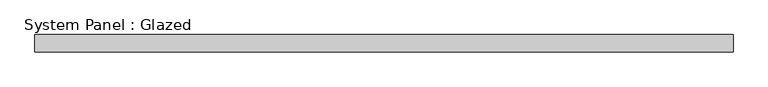
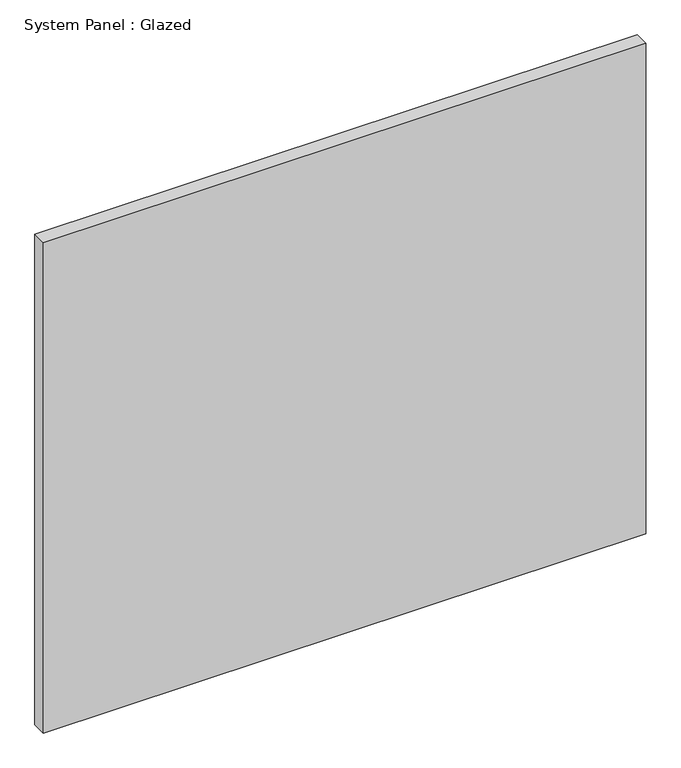
"""IFC4 building model written with IfcOpenShell, lengths in millimetres: plate geometry, System Panel : Glazed."""

from ifc_helpers import new_model, si_unit, origin, origin_with_axes, place, context, project, spatial, polyline, outline, extrude, source, transform, mapped, element, save


def system_panel_glazed_37b2116f(model_context):
    return source(origin(), model_context, "Body", "SweptSolid", [
        extrude(outline(polyline([(517.525, 19.05), (-517.525, 19.05), (-517.525, 44.45), (517.525, 44.45), (517.525, 19.05)])), origin_with_axes(), (0.0, 0.0, 1.0), 890.5158113),
    ])


if __name__ == "__main__":
    model = new_model("IFC4")
    model_context = context("Model", 3, world=origin())
    ifc_project = project(units=[si_unit("LENGTHUNIT", "METRE", prefix="MILLI")], contexts=[model_context])
    site = spatial("IfcSite", under=ifc_project)
    building = spatial("IfcBuilding", under=site)
    placement = place(None, origin())
    system_panel_glazed_shape = system_panel_glazed_37b2116f(model_context)
    element("IfcPlate", 1, ObjectType="System Panel : Glazed", at=placement, inside=building, context=model_context, shape_type="MappedRepresentation", body=[
        mapped(system_panel_glazed_shape, transform((0.0, 0.0, 0.0), x_axis=(1.0, 0.0, 0.0), y_axis=(0.0, 1.0, 0.0), z_axis=(0.0, 0.0, 1.0))),
    ])
    save(model, "model.ifc")

# Revit data of these elements
# Type "System Panel : Glazed"
#   Construction Type Id = "GSP4R"
#   Analytic Construction = "1/8 in Pilkington single glazing"
#   Visual Light Transmittance = 0.9
#   Solar Heat Gain Coefficient = 0.86
#   Heat Transfer Coefficient (U) = 1.18115 BTU/(h·ft²·°F)
#   Define Thermal Properties by = 1
# Element 1 (IfcPlate, "System Panel : Glazed")
#   Materials on its faces: "Glass"
# Materials
#   "Glass": class "Glass", colour RGB 0 128 192, transparency 0.75, Description = "Soda Lime Glass", Cost = 0
